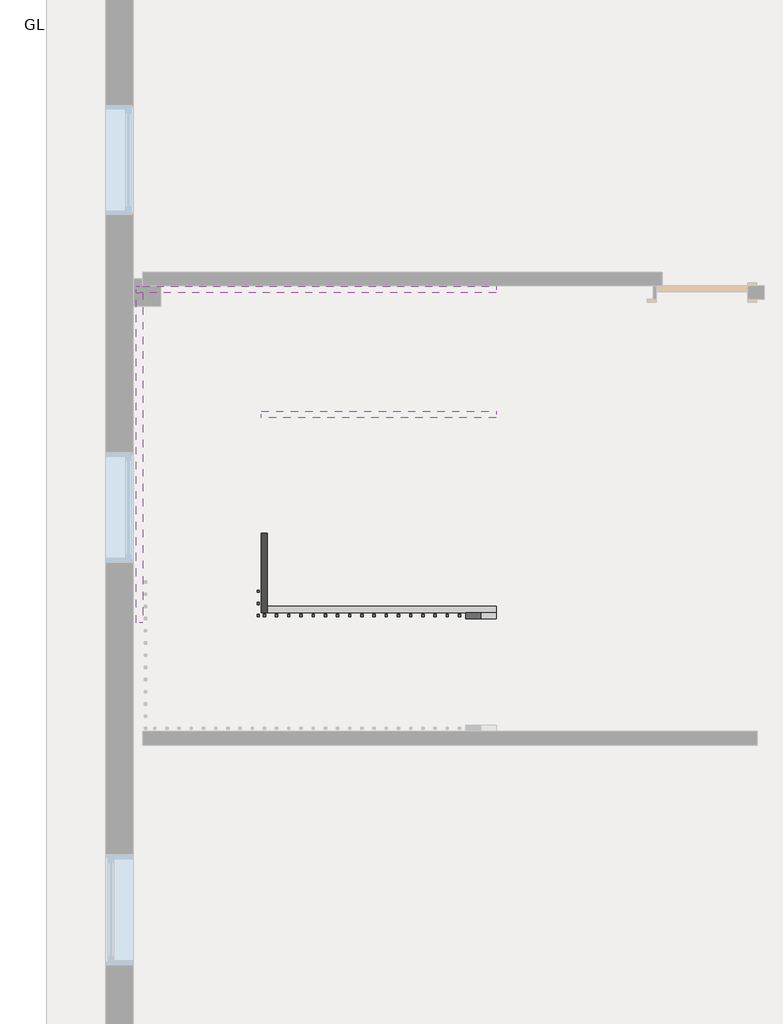
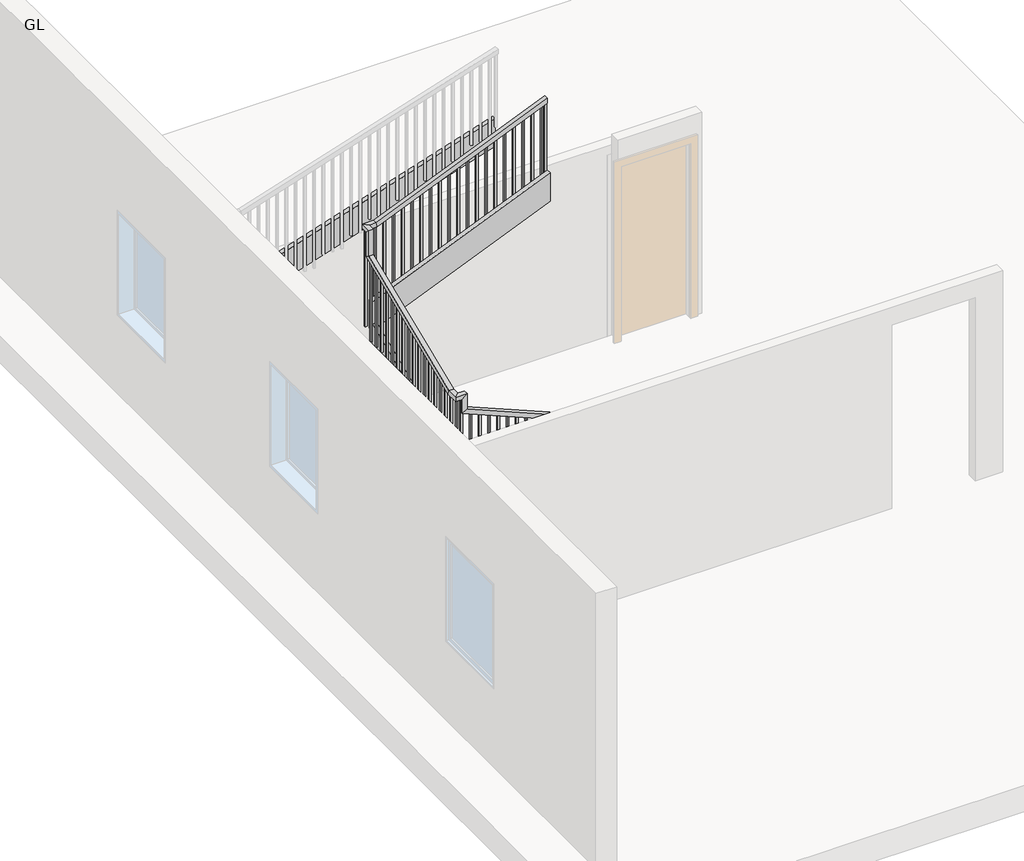
# One storey, part 3 of 3: 6 members, 1 railing.
"""IFC4 building model written with IfcOpenShell, lengths in millimetres."""

from ifc_helpers import new_model, si_unit, frame, origin, place, context, project, spatial, polyline, outline, extrude, faceted_brep, element, save

model = new_model("IFC4")

# Units and contexts
model_context = context("Model", 3, world=origin())
ifc_project = project(units=[si_unit("LENGTHUNIT", "METRE", prefix="MILLI")], contexts=[model_context])

# Site, building, storey
site = spatial("IfcSite", under=ifc_project)
building = spatial("IfcBuilding", under=site)
storey = spatial("IfcBuildingStorey", under=building, Name="GL", Elevation=3200.4)

# Members
placement = place(None, origin())
element("IfcMember", 1, ObjectType="Stringer - 2\" Width", at=placement, inside=storey, context=model_context, shape_type="SweptSolid", body=[
    extrude(outline(polyline([(3200.4, 5202.3334712), (3515.1886477, 5202.3334712), (4142.5719103, 3707.0700288), (4142.5719103, 2919.2768366), (3200.4, 5164.7865561), (3200.4, 5202.3334712)])), frame((0.0, 4060.0450307, 0.0), z_axis=(0.0, 1.0, 0.0), x_axis=(0.0, 0.0, 1.0)), (0.0, 0.0, 1.0), 50.8),
])
element("IfcMember", 2, ObjectType="Stringer - 2\" Width", at=placement, inside=storey, context=model_context, shape_type="SweptSolid", body=[
    extrude(outline(polyline([(5015.4041654, 4420.8977979), (7768.4450307, 5267.9872949), (7768.4450307, 4949.0851248), (6051.8362182, 4420.8977979), (5015.4041654, 4420.8977979)])), frame((2205.1334712, 0.0, 0.0), z_axis=(1.0, 0.0, 0.0), x_axis=(0.0, 1.0, 0.0)), (0.0, 0.0, 1.0), 50.8),
])
element("IfcMember", 3, ObjectType="Stringer - 2\" Width", at=placement, inside=storey, context=model_context, shape_type="SweptSolid", body=[
    extrude(outline(polyline([(5252.2454089, 2205.1334712), (4949.0851248, 2205.1334712), (4949.0851248, 2257.6240611), (5886.3931599, 5202.3334712), (6206.2613241, 5202.3334712), (5252.2454089, 2205.1334712)])), frame((0.0, 7768.4450307, 0.0), z_axis=(0.0, 1.0, 0.0), x_axis=(0.0, 0.0, 1.0)), (0.0, 0.0, 1.0), 50.8),
])
element("IfcMember", 4, ObjectType="Stringer - 2\" Width", at=placement, inside=storey, context=model_context, shape_type="SweptSolid", body=[
    extrude(outline(polyline([(3200.4, 5202.3334712), (3515.1886477, 5202.3334712), (4314.489347, 3297.3334712), (3983.9467489, 3297.3334712), (3200.4, 5164.7865562), (3200.4, 5202.3334712)])), frame((0.0, 5101.4450307, 0.0), z_axis=(0.0, 1.0, 0.0), x_axis=(0.0, 0.0, 1.0)), (0.0, 0.0, 1.0), 50.8),
])
element("IfcMember", 5, ObjectType="Stringer - 2\" Width", at=placement, inside=storey, context=model_context, shape_type="SweptSolid", body=[
    extrude(outline(polyline([(5101.4450307, 4122.4922035), (5101.4450307, 4453.0348016), (6727.0450307, 5135.1047317), (6727.0450307, 4804.5621336), (5101.4450307, 4122.4922035)])), frame((3246.5334712, 0.0, 0.0), z_axis=(1.0, 0.0, 0.0), x_axis=(0.0, 1.0, 0.0)), (0.0, 0.0, 1.0), 50.8),
])
element("IfcMember", 6, ObjectType="Stringer - 2\" Width", at=placement, inside=storey, context=model_context, shape_type="SweptSolid", body=[
    extrude(outline(polyline([(5390.8809554, 3246.5334712), (5060.3383573, 3246.5334712), (5880.9537419, 5202.3334712), (6211.4963401, 5202.3334712), (5390.8809554, 3246.5334712)])), frame((0.0, 6727.0450307, 0.0), z_axis=(0.0, 1.0, 0.0), x_axis=(0.0, 0.0, 1.0)), (0.0, 0.0, 1.0), 50.8),
])

# Railing
element("IfcRailing", 7, ObjectType="Handrail - Rectangular", at=placement, inside=storey, context=model_context, shape_type="SolidModel", body=[
    faceted_brep([(5202.3334712, 5050.6450307, 4349.2615385), (5202.3334712, 5050.6450307, 4294.1711054), (5202.3334712, 5101.4450307, 4294.1711054), (5202.3334712, 5101.4450307, 4349.2615385), (3322.7334712, 5050.6450307, 5137.9048951), (3271.9334712, 5050.6450307, 5104.1291474), (3271.9334712, 5101.4450307, 5104.1291474), (3322.7334712, 5101.4450307, 5137.9048951), (3322.7334712, 5050.6450307, 5319.0797203), (3271.9334712, 5050.6450307, 5268.2797203), (3271.9334712, 5101.4450307, 5268.2797203), (3322.7334712, 5101.4450307, 5319.0797203), (3195.7334712, 5050.6450307, 5319.0797203), (3195.7334712, 5050.6450307, 5268.2797203), (3246.5334712, 5101.4450307, 5268.2797203), (3246.5334712, 5101.4450307, 5319.0797203), (3195.7334712, 5177.6450307, 5319.0797203), (3195.7334712, 5187.8705627, 5268.2797203), (3246.5334712, 5187.8705627, 5268.2797203), (3246.5334712, 5177.6450307, 5319.0797203), (3195.7334712, 6701.6450307, 5958.5202797), (3195.7334712, 6752.4450307, 5924.744532), (3246.5334712, 6752.4450307, 5924.744532), (3246.5334712, 6701.6450307, 5958.5202797), (5202.3334712, 6828.6450307, 7045.5692308), (5202.3334712, 6777.8450307, 7045.5692308), (5202.3334712, 6777.8450307, 6990.4787978), (5202.3334712, 6828.6450307, 6990.4787978), (3332.9590032, 6828.6450307, 6206.1258741), (3322.7334712, 6828.6450307, 6256.9258741), (3332.9590032, 6777.8450307, 6206.1258741), (3322.7334712, 6777.8450307, 6256.9258741), (3195.7334712, 6701.6450307, 6256.9258741), (3195.7334712, 6752.4450307, 6206.1258741), (3246.5334712, 6752.4450307, 6206.1258741), (3246.5334712, 6701.6450307, 6256.9258741), (3195.7334712, 6828.6450307, 6256.9258741), (3195.7334712, 6828.6450307, 6206.1258741), (3246.5334712, 6777.8450307, 6206.1258741), (3246.5334712, 6777.8450307, 6256.9258741)], [[[0, 1, 2, 3]], [[1, 0, 4, 5]], [[2, 1, 5, 6]], [[3, 2, 6, 7]], [[0, 3, 7, 4]], [[5, 4, 8, 9]], [[6, 5, 9, 10]], [[7, 6, 10, 11]], [[4, 7, 11, 8]], [[9, 8, 12, 13]], [[10, 9, 13, 14]], [[11, 10, 14, 15]], [[8, 11, 15, 12]], [[13, 12, 16, 17]], [[14, 13, 17, 18]], [[15, 14, 18, 19]], [[12, 15, 19, 16]], [[17, 16, 20, 21]], [[18, 17, 21, 22]], [[19, 18, 22, 23]], [[16, 19, 23, 20]], [[24, 25, 26, 27]], [[28, 29, 24, 27]], [[30, 28, 27, 26]], [[31, 30, 26, 25]], [[29, 31, 25, 24]], [[21, 20, 32, 33]], [[22, 21, 33, 34]], [[23, 22, 34, 35]], [[20, 23, 35, 32]], [[33, 32, 36, 37]], [[34, 33, 37, 38]], [[35, 34, 38, 39]], [[32, 35, 39, 36]], [[37, 36, 29, 28]], [[38, 37, 28, 30]], [[39, 38, 30, 31]], [[36, 39, 31, 29]]]),
    extrude(outline(polyline([(6973.1606159, 5161.0584712), (6965.1676089, 5142.0084712), (6013.9384615, 5142.0084712), (6013.9384615, 5161.0584712), (6973.1606159, 5161.0584712)])), frame((0.0, 6793.7200307, 0.0), z_axis=(0.0, 1.0, 0.0), x_axis=(0.0, 0.0, 1.0)), (0.0, 0.0, 1.0), 19.05),
    extrude(outline(polyline([(6930.5312453, 5059.4584712), (6922.5382383, 5040.4084712), (6013.9384615, 5040.4084712), (6013.9384615, 5059.4584712), (6930.5312453, 5059.4584712)])), frame((0.0, 6793.7200307, 0.0), z_axis=(0.0, 1.0, 0.0), x_axis=(0.0, 0.0, 1.0)), (0.0, 0.0, 1.0), 19.05),
    extrude(outline(polyline([(6887.9018747, 4957.8584712), (6879.9088677, 4938.8084712), (6013.9384615, 4938.8084712), (6013.9384615, 4957.8584712), (6887.9018747, 4957.8584712)])), frame((0.0, 6793.7200307, 0.0), z_axis=(0.0, 1.0, 0.0), x_axis=(0.0, 0.0, 1.0)), (0.0, 0.0, 1.0), 19.05),
    extrude(outline(polyline([(6845.272504, 4856.2584712), (6837.2794971, 4837.2084712), (5896.7076923, 4837.2084712), (5896.7076923, 4856.2584712), (6845.272504, 4856.2584712)])), frame((0.0, 6793.7200307, 0.0), z_axis=(0.0, 1.0, 0.0), x_axis=(0.0, 0.0, 1.0)), (0.0, 0.0, 1.0), 19.05),
    extrude(outline(polyline([(6802.6431334, 4754.6584712), (6794.6501264, 4735.6084712), (5896.7076923, 4735.6084712), (5896.7076923, 4754.6584712), (6802.6431334, 4754.6584712)])), frame((0.0, 6793.7200307, 0.0), z_axis=(0.0, 1.0, 0.0), x_axis=(0.0, 0.0, 1.0)), (0.0, 0.0, 1.0), 19.05),
    extrude(outline(polyline([(6760.0137628, 4653.0584712), (6752.0207558, 4634.0084712), (5896.7076923, 4634.0084712), (5896.7076923, 4653.0584712), (6760.0137628, 4653.0584712)])), frame((0.0, 6793.7200307, 0.0), z_axis=(0.0, 1.0, 0.0), x_axis=(0.0, 0.0, 1.0)), (0.0, 0.0, 1.0), 19.05),
    extrude(outline(polyline([(6717.3843922, 4551.4584712), (6709.3913852, 4532.4084712), (5779.4769231, 4532.4084712), (5779.4769231, 4551.4584712), (6717.3843922, 4551.4584712)])), frame((0.0, 6793.7200307, 0.0), z_axis=(0.0, 1.0, 0.0), x_axis=(0.0, 0.0, 1.0)), (0.0, 0.0, 1.0), 19.05),
    extrude(outline(polyline([(6674.7550215, 4449.8584712), (6666.7620145, 4430.8084712), (5779.4769231, 4430.8084712), (5779.4769231, 4449.8584712), (6674.7550215, 4449.8584712)])), frame((0.0, 6793.7200307, 0.0), z_axis=(0.0, 1.0, 0.0), x_axis=(0.0, 0.0, 1.0)), (0.0, 0.0, 1.0), 19.05),
    extrude(outline(polyline([(6632.1256509, 4348.2584712), (6624.1326439, 4329.2084712), (5662.2461538, 4329.2084712), (5662.2461538, 4348.2584712), (6632.1256509, 4348.2584712)])), frame((0.0, 6793.7200307, 0.0), z_axis=(0.0, 1.0, 0.0), x_axis=(0.0, 0.0, 1.0)), (0.0, 0.0, 1.0), 19.05),
    extrude(outline(polyline([(6589.4962803, 4246.6584712), (6581.5032733, 4227.6084712), (5662.2461538, 4227.6084712), (5662.2461538, 4246.6584712), (6589.4962803, 4246.6584712)])), frame((0.0, 6793.7200307, 0.0), z_axis=(0.0, 1.0, 0.0), x_axis=(0.0, 0.0, 1.0)), (0.0, 0.0, 1.0), 19.05),
    extrude(outline(polyline([(6546.8669096, 4145.0584712), (6538.8739026, 4126.0084712), (5662.2461538, 4126.0084712), (5662.2461538, 4145.0584712), (6546.8669096, 4145.0584712)])), frame((0.0, 6793.7200307, 0.0), z_axis=(0.0, 1.0, 0.0), x_axis=(0.0, 0.0, 1.0)), (0.0, 0.0, 1.0), 19.05),
    extrude(outline(polyline([(6504.237539, 4043.4584712), (6496.244532, 4024.4084712), (5545.0153846, 4024.4084712), (5545.0153846, 4043.4584712), (6504.237539, 4043.4584712)])), frame((0.0, 6793.7200307, 0.0), z_axis=(0.0, 1.0, 0.0), x_axis=(0.0, 0.0, 1.0)), (0.0, 0.0, 1.0), 19.05),
    extrude(outline(polyline([(6461.6081684, 3941.8584712), (6453.6151614, 3922.8084712), (5545.0153846, 3922.8084712), (5545.0153846, 3941.8584712), (6461.6081684, 3941.8584712)])), frame((0.0, 6793.7200307, 0.0), z_axis=(0.0, 1.0, 0.0), x_axis=(0.0, 0.0, 1.0)), (0.0, 0.0, 1.0), 19.05),
    extrude(outline(polyline([(6418.9787978, 3840.2584712), (6410.9857908, 3821.2084712), (5545.0153846, 3821.2084712), (5545.0153846, 3840.2584712), (6418.9787978, 3840.2584712)])), frame((0.0, 6793.7200307, 0.0), z_axis=(0.0, 1.0, 0.0), x_axis=(0.0, 0.0, 1.0)), (0.0, 0.0, 1.0), 19.05),
    extrude(outline(polyline([(6376.3494271, 3738.6584712), (6368.3564201, 3719.6084712), (5427.7846154, 3719.6084712), (5427.7846154, 3738.6584712), (6376.3494271, 3738.6584712)])), frame((0.0, 6793.7200307, 0.0), z_axis=(0.0, 1.0, 0.0), x_axis=(0.0, 0.0, 1.0)), (0.0, 0.0, 1.0), 19.05),
    extrude(outline(polyline([(6333.7200565, 3637.0584712), (6325.7270495, 3618.0084712), (5427.7846154, 3618.0084712), (5427.7846154, 3637.0584712), (6333.7200565, 3637.0584712)])), frame((0.0, 6793.7200307, 0.0), z_axis=(0.0, 1.0, 0.0), x_axis=(0.0, 0.0, 1.0)), (0.0, 0.0, 1.0), 19.05),
    extrude(outline(polyline([(6291.0906859, 3535.4584712), (6283.0976789, 3516.4084712), (5427.7846154, 3516.4084712), (5427.7846154, 3535.4584712), (6291.0906859, 3535.4584712)])), frame((0.0, 6793.7200307, 0.0), z_axis=(0.0, 1.0, 0.0), x_axis=(0.0, 0.0, 1.0)), (0.0, 0.0, 1.0), 19.05),
    extrude(outline(polyline([(6248.4613152, 3433.8584712), (6240.4683082, 3414.8084712), (5310.5538462, 3414.8084712), (5310.5538462, 3433.8584712), (6248.4613152, 3433.8584712)])), frame((0.0, 6793.7200307, 0.0), z_axis=(0.0, 1.0, 0.0), x_axis=(0.0, 0.0, 1.0)), (0.0, 0.0, 1.0), 19.05),
    extrude(outline(polyline([(6205.8319446, 3332.2584712), (6197.8389376, 3313.2084712), (5310.5538462, 3313.2084712), (5310.5538462, 3332.2584712), (6205.8319446, 3332.2584712)])), frame((0.0, 6793.7200307, 0.0), z_axis=(0.0, 1.0, 0.0), x_axis=(0.0, 0.0, 1.0)), (0.0, 0.0, 1.0), 19.05),
    extrude(outline(polyline([(6692.1200307, 5899.4333432), (6711.1700307, 5907.4263502), (6711.1700307, 4958.8615385), (6692.1200307, 4958.8615385), (6692.1200307, 5899.4333432)])), frame((3211.6084712, 0.0, 0.0), z_axis=(1.0, 0.0, 0.0), x_axis=(0.0, 1.0, 0.0)), (0.0, 0.0, 1.0), 19.05),
    extrude(outline(polyline([(6590.5200307, 5856.8039726), (6609.5700307, 5864.7969796), (6609.5700307, 4958.8615385), (6590.5200307, 4958.8615385), (6590.5200307, 5856.8039726)])), frame((3211.6084712, 0.0, 0.0), z_axis=(1.0, 0.0, 0.0), x_axis=(0.0, 1.0, 0.0)), (0.0, 0.0, 1.0), 19.05),
    extrude(outline(polyline([(6488.9200307, 5814.1746019), (6507.9700307, 5822.1676089), (6507.9700307, 4958.8615385), (6488.9200307, 4958.8615385), (6488.9200307, 5814.1746019)])), frame((3211.6084712, 0.0, 0.0), z_axis=(1.0, 0.0, 0.0), x_axis=(0.0, 1.0, 0.0)), (0.0, 0.0, 1.0), 19.05),
    extrude(outline(polyline([(6387.3200307, 5771.5452313), (6406.3700307, 5779.5382383), (6406.3700307, 4841.6307692), (6387.3200307, 4841.6307692), (6387.3200307, 5771.5452313)])), frame((3211.6084712, 0.0, 0.0), z_axis=(1.0, 0.0, 0.0), x_axis=(0.0, 1.0, 0.0)), (0.0, 0.0, 1.0), 19.05),
    extrude(outline(polyline([(6285.7200307, 5728.9158607), (6304.7700307, 5736.9088677), (6304.7700307, 4841.6307692), (6285.7200307, 4841.6307692), (6285.7200307, 5728.9158607)])), frame((3211.6084712, 0.0, 0.0), z_axis=(1.0, 0.0, 0.0), x_axis=(0.0, 1.0, 0.0)), (0.0, 0.0, 1.0), 19.05),
    extrude(outline(polyline([(6184.1200307, 5686.2864901), (6203.1700307, 5694.2794971), (6203.1700307, 4724.4), (6184.1200307, 4724.4), (6184.1200307, 5686.2864901)])), frame((3211.6084712, 0.0, 0.0), z_axis=(1.0, 0.0, 0.0), x_axis=(0.0, 1.0, 0.0)), (0.0, 0.0, 1.0), 19.05),
    extrude(outline(polyline([(6082.5200307, 5643.6571194), (6101.5700307, 5651.6501264), (6101.5700307, 4724.4), (6082.5200307, 4724.4), (6082.5200307, 5643.6571194)])), frame((3211.6084712, 0.0, 0.0), z_axis=(1.0, 0.0, 0.0), x_axis=(0.0, 1.0, 0.0)), (0.0, 0.0, 1.0), 19.05),
    extrude(outline(polyline([(5980.9200307, 5601.0277488), (5999.9700307, 5609.0207558), (5999.9700307, 4724.4), (5980.9200307, 4724.4), (5980.9200307, 5601.0277488)])), frame((3211.6084712, 0.0, 0.0), z_axis=(1.0, 0.0, 0.0), x_axis=(0.0, 1.0, 0.0)), (0.0, 0.0, 1.0), 19.05),
    extrude(outline(polyline([(5879.3200307, 5558.3983782), (5898.3700307, 5566.3913852), (5898.3700307, 4607.1692308), (5879.3200307, 4607.1692308), (5879.3200307, 5558.3983782)])), frame((3211.6084712, 0.0, 0.0), z_axis=(1.0, 0.0, 0.0), x_axis=(0.0, 1.0, 0.0)), (0.0, 0.0, 1.0), 19.05),
    extrude(outline(polyline([(5777.7200307, 5515.7690075), (5796.7700307, 5523.7620145), (5796.7700307, 4607.1692308), (5777.7200307, 4607.1692308), (5777.7200307, 5515.7690075)])), frame((3211.6084712, 0.0, 0.0), z_axis=(1.0, 0.0, 0.0), x_axis=(0.0, 1.0, 0.0)), (0.0, 0.0, 1.0), 19.05),
    extrude(outline(polyline([(5676.1200307, 5473.1396369), (5695.1700307, 5481.1326439), (5695.1700307, 4607.1692308), (5676.1200307, 4607.1692308), (5676.1200307, 5473.1396369)])), frame((3211.6084712, 0.0, 0.0), z_axis=(1.0, 0.0, 0.0), x_axis=(0.0, 1.0, 0.0)), (0.0, 0.0, 1.0), 19.05),
    extrude(outline(polyline([(5574.5200307, 5430.5102663), (5593.5700307, 5438.5032733), (5593.5700307, 4489.9384615), (5574.5200307, 4489.9384615), (5574.5200307, 5430.5102663)])), frame((3211.6084712, 0.0, 0.0), z_axis=(1.0, 0.0, 0.0), x_axis=(0.0, 1.0, 0.0)), (0.0, 0.0, 1.0), 19.05),
    extrude(outline(polyline([(5472.9200307, 5387.8808957), (5491.9700307, 5395.8739026), (5491.9700307, 4489.9384615), (5472.9200307, 4489.9384615), (5472.9200307, 5387.8808957)])), frame((3211.6084712, 0.0, 0.0), z_axis=(1.0, 0.0, 0.0), x_axis=(0.0, 1.0, 0.0)), (0.0, 0.0, 1.0), 19.05),
    extrude(outline(polyline([(5371.3200307, 5345.251525), (5390.3700307, 5353.244532), (5390.3700307, 4489.9384615), (5371.3200307, 4489.9384615), (5371.3200307, 5345.251525)])), frame((3211.6084712, 0.0, 0.0), z_axis=(1.0, 0.0, 0.0), x_axis=(0.0, 1.0, 0.0)), (0.0, 0.0, 1.0), 19.05),
    extrude(outline(polyline([(5269.7200307, 5302.6221544), (5288.7700307, 5310.6151614), (5288.7700307, 4372.7076923), (5269.7200307, 4372.7076923), (5269.7200307, 5302.6221544)])), frame((3211.6084712, 0.0, 0.0), z_axis=(1.0, 0.0, 0.0), x_axis=(0.0, 1.0, 0.0)), (0.0, 0.0, 1.0), 19.05),
    extrude(outline(polyline([(5168.1200307, 5259.9927838), (5187.1700307, 5267.9857908), (5187.1700307, 4372.7076923), (5168.1200307, 4372.7076923), (5168.1200307, 5259.9927838)])), frame((3211.6084712, 0.0, 0.0), z_axis=(1.0, 0.0, 0.0), x_axis=(0.0, 1.0, 0.0)), (0.0, 0.0, 1.0), 19.05),
    extrude(outline(polyline([(3281.4584712, 5085.5700307), (3281.4584712, 5066.5200307), (3262.4084712, 5066.5200307), (3262.4084712, 5085.5700307), (3281.4584712, 5085.5700307)])), frame((0.0, 0.0, 4138.2461538), z_axis=(0.0, 0.0, 1.0), x_axis=(1.0, 0.0, 0.0)), (0.0, 0.0, 1.0), 1130.0335664),
    extrude(outline(polyline([(5057.5032733, 3383.0584712), (5065.4962803, 3364.0084712), (4138.2461538, 3364.0084712), (4138.2461538, 3383.0584712), (5057.5032733, 3383.0584712)])), frame((0.0, 5066.5200307, 0.0), z_axis=(0.0, 1.0, 0.0), x_axis=(0.0, 0.0, 1.0)), (0.0, 0.0, 1.0), 19.05),
    extrude(outline(polyline([(5014.8739026, 3484.6584712), (5022.8669096, 3465.6084712), (4138.2461538, 3465.6084712), (4138.2461538, 3484.6584712), (5014.8739026, 3484.6584712)])), frame((0.0, 5066.5200307, 0.0), z_axis=(0.0, 1.0, 0.0), x_axis=(0.0, 0.0, 1.0)), (0.0, 0.0, 1.0), 19.05),
    extrude(outline(polyline([(4972.244532, 3586.2584712), (4980.237539, 3567.2084712), (4021.0153846, 3567.2084712), (4021.0153846, 3586.2584712), (4972.244532, 3586.2584712)])), frame((0.0, 5066.5200307, 0.0), z_axis=(0.0, 1.0, 0.0), x_axis=(0.0, 0.0, 1.0)), (0.0, 0.0, 1.0), 19.05),
    extrude(outline(polyline([(4929.6151614, 3687.8584712), (4937.6081684, 3668.8084712), (4021.0153846, 3668.8084712), (4021.0153846, 3687.8584712), (4929.6151614, 3687.8584712)])), frame((0.0, 5066.5200307, 0.0), z_axis=(0.0, 1.0, 0.0), x_axis=(0.0, 0.0, 1.0)), (0.0, 0.0, 1.0), 19.05),
    extrude(outline(polyline([(4886.9857908, 3789.4584712), (4894.9787978, 3770.4084712), (4021.0153846, 3770.4084712), (4021.0153846, 3789.4584712), (4886.9857908, 3789.4584712)])), frame((0.0, 5066.5200307, 0.0), z_axis=(0.0, 1.0, 0.0), x_axis=(0.0, 0.0, 1.0)), (0.0, 0.0, 1.0), 19.05),
    extrude(outline(polyline([(4844.3564201, 3891.0584712), (4852.3494271, 3872.0084712), (3903.7846154, 3872.0084712), (3903.7846154, 3891.0584712), (4844.3564201, 3891.0584712)])), frame((0.0, 5066.5200307, 0.0), z_axis=(0.0, 1.0, 0.0), x_axis=(0.0, 0.0, 1.0)), (0.0, 0.0, 1.0), 19.05),
    extrude(outline(polyline([(4801.7270495, 3992.6584712), (4809.7200565, 3973.6084712), (3903.7846154, 3973.6084712), (3903.7846154, 3992.6584712), (4801.7270495, 3992.6584712)])), frame((0.0, 5066.5200307, 0.0), z_axis=(0.0, 1.0, 0.0), x_axis=(0.0, 0.0, 1.0)), (0.0, 0.0, 1.0), 19.05),
    extrude(outline(polyline([(4759.0976789, 4094.2584712), (4767.0906859, 4075.2084712), (3903.7846154, 4075.2084712), (3903.7846154, 4094.2584712), (4759.0976789, 4094.2584712)])), frame((0.0, 5066.5200307, 0.0), z_axis=(0.0, 1.0, 0.0), x_axis=(0.0, 0.0, 1.0)), (0.0, 0.0, 1.0), 19.05),
    extrude(outline(polyline([(4716.4683082, 4195.8584712), (4724.4613152, 4176.8084712), (3786.5538462, 4176.8084712), (3786.5538462, 4195.8584712), (4716.4683082, 4195.8584712)])), frame((0.0, 5066.5200307, 0.0), z_axis=(0.0, 1.0, 0.0), x_axis=(0.0, 0.0, 1.0)), (0.0, 0.0, 1.0), 19.05),
    extrude(outline(polyline([(4673.8389376, 4297.4584712), (4681.8319446, 4278.4084712), (3786.5538462, 4278.4084712), (3786.5538462, 4297.4584712), (4673.8389376, 4297.4584712)])), frame((0.0, 5066.5200307, 0.0), z_axis=(0.0, 1.0, 0.0), x_axis=(0.0, 0.0, 1.0)), (0.0, 0.0, 1.0), 19.05),
    extrude(outline(polyline([(4631.209567, 4399.0584712), (4639.202574, 4380.0084712), (3669.3230769, 4380.0084712), (3669.3230769, 4399.0584712), (4631.209567, 4399.0584712)])), frame((0.0, 5066.5200307, 0.0), z_axis=(0.0, 1.0, 0.0), x_axis=(0.0, 0.0, 1.0)), (0.0, 0.0, 1.0), 19.05),
    extrude(outline(polyline([(4588.5801964, 4500.6584712), (4596.5732033, 4481.6084712), (3669.3230769, 4481.6084712), (3669.3230769, 4500.6584712), (4588.5801964, 4500.6584712)])), frame((0.0, 5066.5200307, 0.0), z_axis=(0.0, 1.0, 0.0), x_axis=(0.0, 0.0, 1.0)), (0.0, 0.0, 1.0), 19.05),
    extrude(outline(polyline([(4545.9508257, 4602.2584712), (4553.9438327, 4583.2084712), (3669.3230769, 4583.2084712), (3669.3230769, 4602.2584712), (4545.9508257, 4602.2584712)])), frame((0.0, 5066.5200307, 0.0), z_axis=(0.0, 1.0, 0.0), x_axis=(0.0, 0.0, 1.0)), (0.0, 0.0, 1.0), 19.05),
    extrude(outline(polyline([(4503.3214551, 4703.8584712), (4511.3144621, 4684.8084712), (3552.0923077, 4684.8084712), (3552.0923077, 4703.8584712), (4503.3214551, 4703.8584712)])), frame((0.0, 5066.5200307, 0.0), z_axis=(0.0, 1.0, 0.0), x_axis=(0.0, 0.0, 1.0)), (0.0, 0.0, 1.0), 19.05),
    extrude(outline(polyline([(4460.6920845, 4805.4584712), (4468.6850915, 4786.4084712), (3552.0923077, 4786.4084712), (3552.0923077, 4805.4584712), (4460.6920845, 4805.4584712)])), frame((0.0, 5066.5200307, 0.0), z_axis=(0.0, 1.0, 0.0), x_axis=(0.0, 0.0, 1.0)), (0.0, 0.0, 1.0), 19.05),
    extrude(outline(polyline([(4418.0627138, 4907.0584712), (4426.0557208, 4888.0084712), (3552.0923077, 4888.0084712), (3552.0923077, 4907.0584712), (4418.0627138, 4907.0584712)])), frame((0.0, 5066.5200307, 0.0), z_axis=(0.0, 1.0, 0.0), x_axis=(0.0, 0.0, 1.0)), (0.0, 0.0, 1.0), 19.05),
    extrude(outline(polyline([(4375.4333432, 5008.6584712), (4383.4263502, 4989.6084712), (3434.8615385, 4989.6084712), (3434.8615385, 5008.6584712), (4375.4333432, 5008.6584712)])), frame((0.0, 5066.5200307, 0.0), z_axis=(0.0, 1.0, 0.0), x_axis=(0.0, 0.0, 1.0)), (0.0, 0.0, 1.0), 19.05),
    extrude(outline(polyline([(4332.8039726, 5110.2584712), (4340.7969796, 5091.2084712), (3434.8615385, 5091.2084712), (3434.8615385, 5110.2584712), (4332.8039726, 5110.2584712)])), frame((0.0, 5066.5200307, 0.0), z_axis=(0.0, 1.0, 0.0), x_axis=(0.0, 0.0, 1.0)), (0.0, 0.0, 1.0), 19.05),
    extrude(outline(polyline([(3230.6584712, 6793.7200307), (3211.6084712, 6793.7200307), (3211.6084712, 6812.7700307), (3230.6584712, 6812.7700307), (3230.6584712, 6793.7200307)])), frame((0.0, 0.0, 5076.0923077), z_axis=(0.0, 0.0, 1.0), x_axis=(1.0, 0.0, 0.0)), (0.0, 0.0, 1.0), 1130.0335664),
    extrude(outline(polyline([(3230.6584712, 5085.5700307), (3230.6584712, 5066.5200307), (3211.6084712, 5066.5200307), (3211.6084712, 5085.5700307), (3230.6584712, 5085.5700307)])), frame((0.0, 0.0, 4255.4769231), z_axis=(0.0, 0.0, 1.0), x_axis=(1.0, 0.0, 0.0)), (0.0, 0.0, 1.0), 1012.8027972),
    extrude(outline(polyline([(6990.4787978, 5202.3334712), (6982.4857908, 5183.2834712), (6131.1692308, 5183.2834712), (6131.1692308, 5202.3334712), (6990.4787978, 5202.3334712)])), frame((0.0, 6793.7200307, 0.0), z_axis=(0.0, 1.0, 0.0), x_axis=(0.0, 0.0, 1.0)), (0.0, 0.0, 1.0), 19.05),
    extrude(outline(polyline([(4294.1711054, 5202.3334712), (4302.1641124, 5183.2834712), (3317.6307692, 5183.2834712), (3317.6307692, 5202.3334712), (4294.1711054, 5202.3334712)])), frame((0.0, 5066.5200307, 0.0), z_axis=(0.0, 1.0, 0.0), x_axis=(0.0, 0.0, 1.0)), (0.0, 0.0, 1.0), 19.05),
])

save(model, "model.ifc")

# Revit data of these elements
# Type "Handrail - Rectangular"
#   Assembly Code = "C2010400"
#   built-in parameter 1008612 = 0.0416667 (stored number, unit not read)
#   built-in parameter 1008611 = 0.0416667 (stored number, unit not read)
#   built-in parameter 1008609 = 0.333333 (stored number, unit not read)
#   built-in parameter 1008604 = 0.166667 (stored number, unit not read)
#   built-in parameter 1008603 = 0.166667 (stored number, unit not read)
#   Railing Height = 3' - 0"
#   built-in parameter 1008630 = 2
#   built-in parameter 1008610 = 2
#   built-in parameter 1008618 = Baluster - Square : 3/4"
# Elements 1, 2, 3, 4, 5, 6 (IfcMember, "Stringer - 2\" Width")
#   Phase Created = New Construction
# Element 7 (IfcRailing, "Handrail - Rectangular")
#   Phase Created = New Construction
